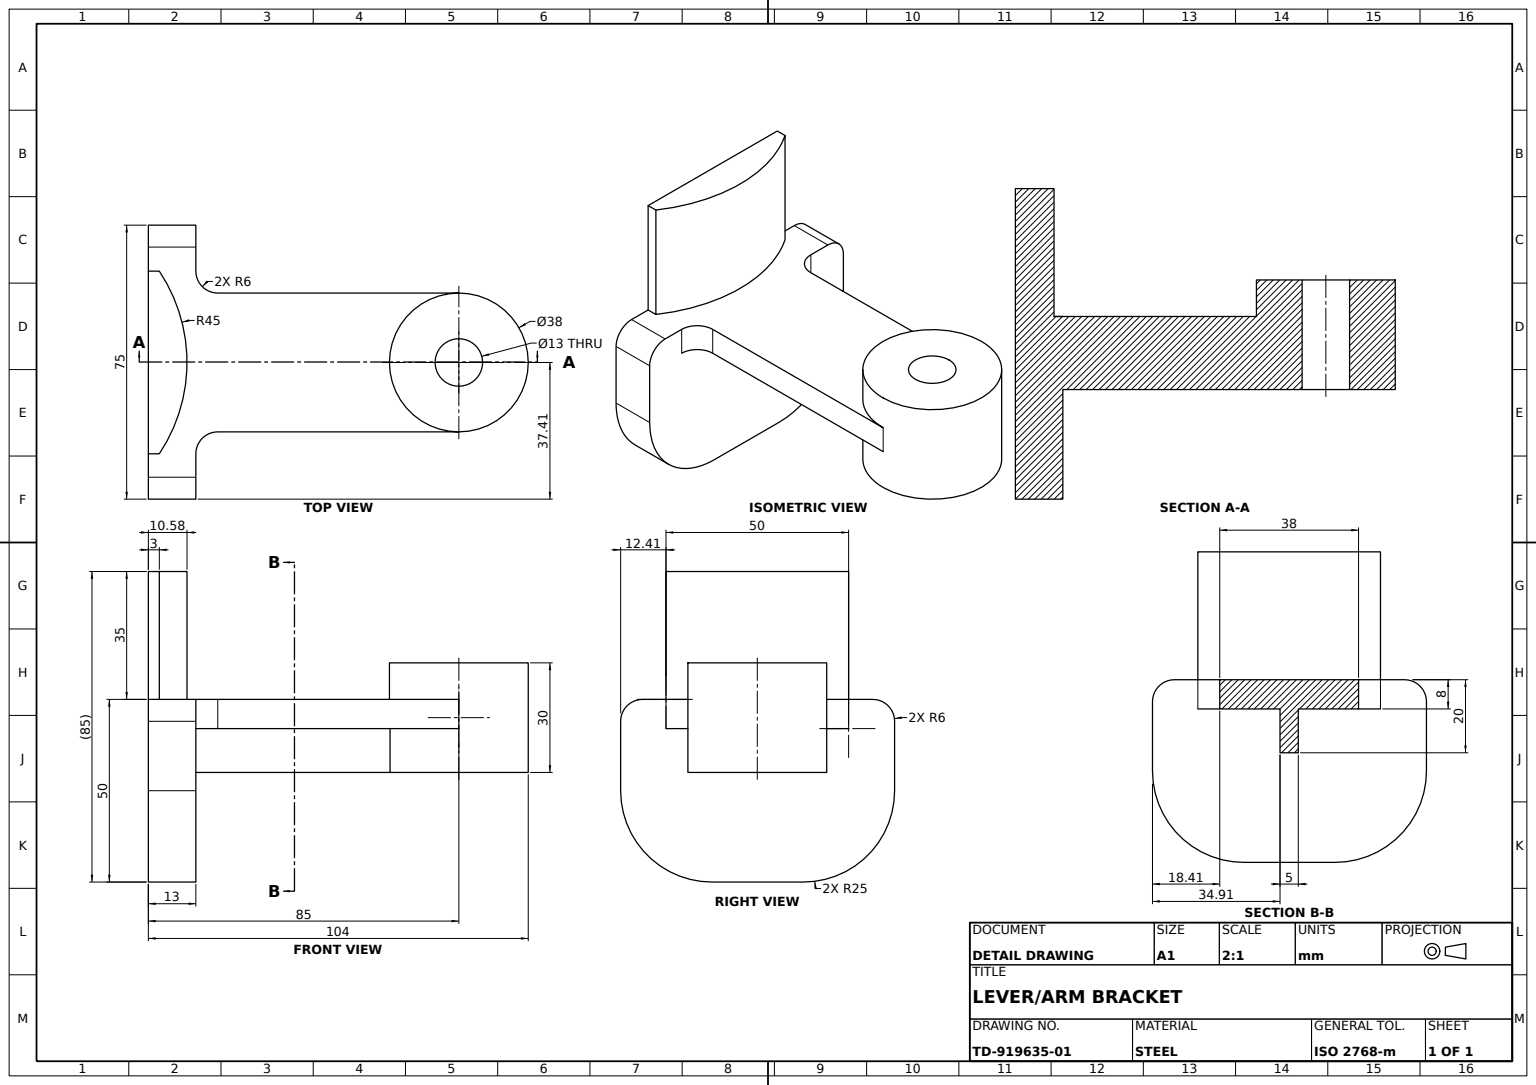
SolidWorks part; units mm, degrees
material "Plain Carbon Steel"
ref_plane "Front Plane" through (0, 0, 0) normal (0, 0, 1) x (1, 0, 0)
ref_plane "Top Plane" through (0, 0, 0) normal (0, 1, 0) x (1, 0, 0)
ref_plane "Right Plane" through (0, 0, 0) normal (1, 0, 0) x (0, 0, -1)
sketch "Base Block Sketch" plane through (0, 0, 0) normal (0, 0, 1) x (1, 0, 0)
  line L9 (0, 0) -> (13, 0)
  line L10 (0, 0) -> (0, 50)
  line L11 (0, 50) -> (13, 50)
  line L12 (13, 0) -> (13, 50)
  dimension "D1" = 13
  dimension "D2" = 50
extrude "Base Block" add sketch "Base Block Sketch" against normal blind 75
fillet "Base End Round R25" radius 25 2 edges at (6.5, 0, -75) (6.5, 0, 0)
fillet "Base Edge Fillet R6" radius 6 2 edges at (6.5, 50, -75) (6.5, 50, 0)
sketch "Arm Web Sketch" plane through (0, 50, 0) normal (0, 1, 0) x (1, 0, 0)
  line L0 (0, 62.4129) -> (0, 12.4129)
  line L1 (0, 37.4129) -> (0, 62.4129)
  line L2 (0, 62.4129) -> (3, 62.4129)
  line L3 (0, 37.4129) -> (0, 12.4129)
  line L4 (0, 12.4129) -> (3, 12.4129)
  arc A0 (3, 12.4129) -> (3, 62.4129) centre (-34.4166, 37.4129) ccw
  line M6 (0, 69) -> (0, 6)
  dimension "D4" = 37.4129
  dimension "D1" = 50
  dimension "D2" = 3
  dimension "D3" = 3
  dimension "D5" = 34.4166
extrude "Arm Web" add sketch "Arm Web Sketch" along normal blind 35 contours L4 A0 L2 L0 M6
ref_plane "Plane1" through (0, 30, 0) normal (0, 1, 0) x (1, 0, 0)
sketch "Hub Boss Sketch" plane through (0, 30, 0) normal (0, 1, 0) x (1, 0, 0)
  line L0 (0, 37.4129) -> (85, 37.4129)
  line L1 (0, 62.4129) -> (0, 12.4129) construction
  circle A0 centre (85, 37.4129) radius 6.5
  circle A1 centre (85, 37.4129) radius 19
  dimension "D2" = 38
  dimension "D3" = 13
  dimension "D1" = 85
extrude "Hub Boss" add sketch "Hub Boss Sketch" along normal blind 30 separate body
ref_plane "Plane2" through (0, 50, 0) normal (0, 1, 0) x (1, 0, 0)
sketch "Upper Lug Sketch" plane through (0, 50, 0) normal (0, 1, 0) x (1, 0, 0)
  line L2 (85, 56.4129) -> (13, 56.4129)
  line L3 (13, 69) -> (13, 6) construction
  line L4 (85, 18.4129) -> (13, 18.4129)
  line L5 (13, 56.4129) -> (13, 18.4129)
  circle A0 centre (85, 37.4129) radius 19 construction
  arc A1 (85, 56.4129) -> (85, 18.4129) centre (85, 37.4129) ccw
extrude "Upper Lug" add sketch "Upper Lug Sketch" against normal blind 8
sketch "Curved Blade Sketch" plane through (0, 50, 0) normal (0, 1, 0) x (1, 0, 0)
  line L2 (0, 34.9129) -> (66.1652, 34.9129)
  line L3 (0, 39.9129) -> (66.1652, 39.9129)
  line L4 (0, 39.9129) -> (0, 34.9129)
  arc A0 (66.1652, 39.9129) -> (66.1652, 34.9129) centre (85, 37.4129) ccw
  dimension "D1" = 19
  dimension "D2" = 5
  dimension "D3" = 2.5
extrude "Curved Blade" add sketch "Curved Blade Sketch" against normal blind 20
fillet "Lug Fillet R6 A" radius 6 1 edges at (13, 46, -18.4129)
fillet "Lug Fillet R6 B" radius 6 1 edges at (13, 46, -56.4129)
